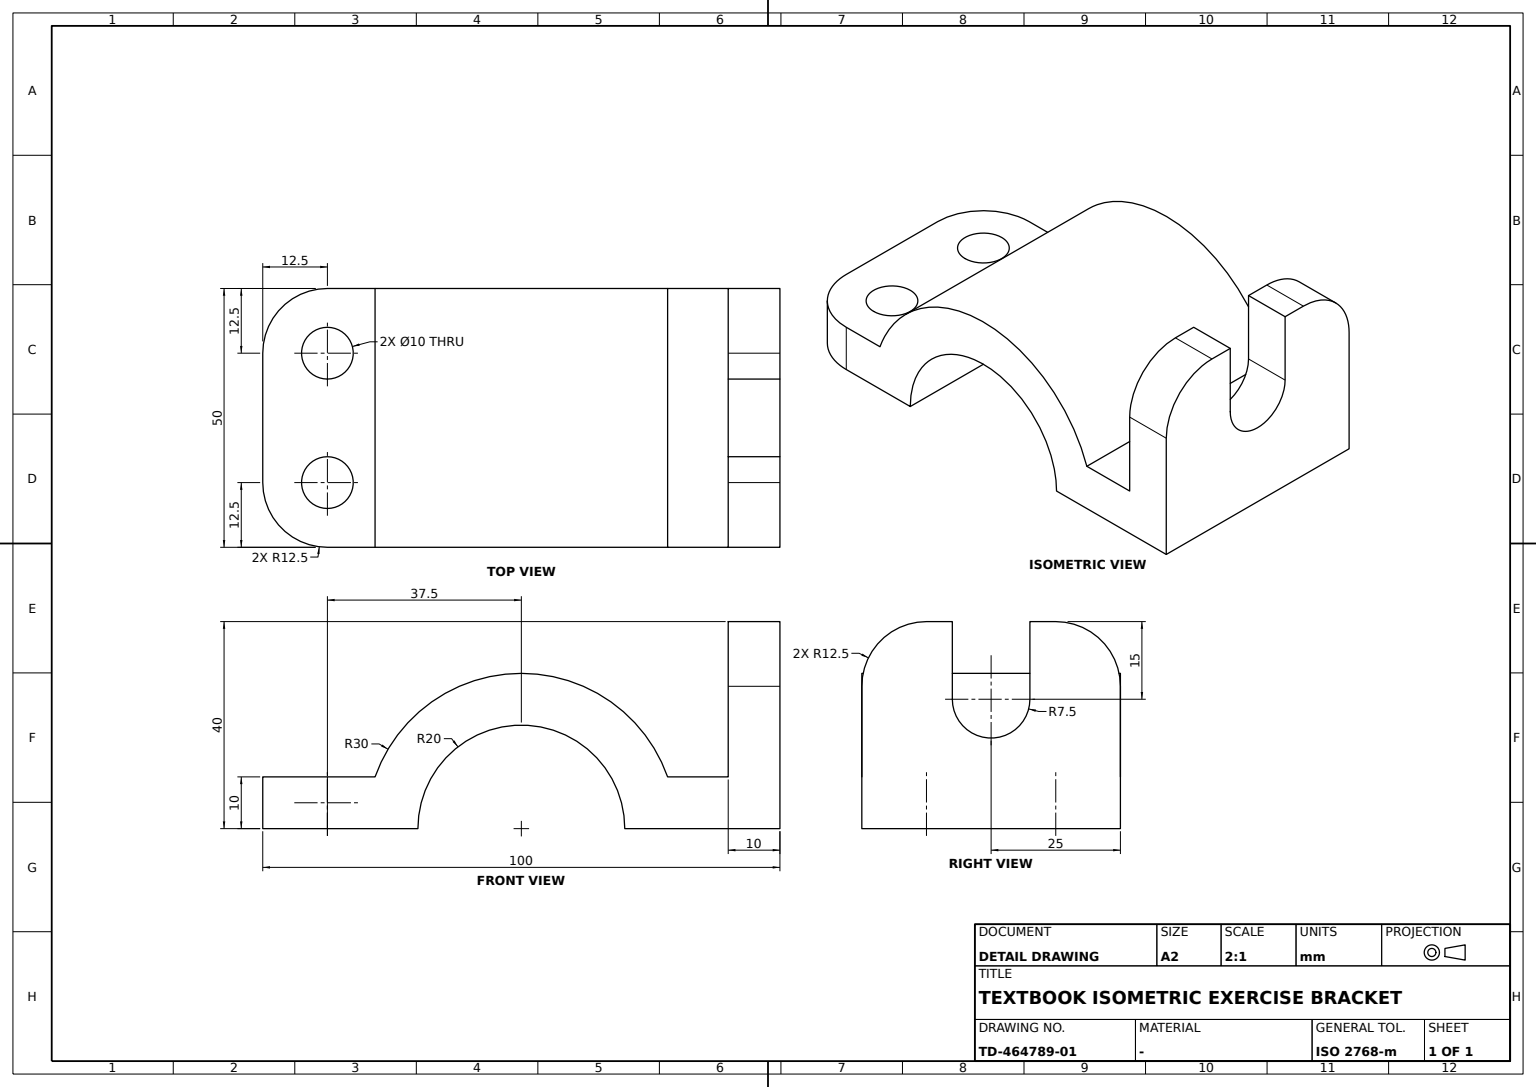
CATIA V5 part; units mm, degrees
sketch "Sketch1" plane through (0, 0, 0) normal (1, 0, 0) x (0, 1, 0)
  line L0 (-20, 0) -> (20, 0) construction
  point P0 (-20, 0)
  point P1 (20, 0)
  arc A0 (20, 0) -> (-20, 0) centre (0, 0) ccw
  point P2 (20, 0)
  point P3 (-20, 0)
  line L1 (20, 0) -> (50, 0)
  point P4 (50, 0)
  line L2 (-20, 0) -> (-50, 0)
  point P5 (-50, 0)
  line L3 (-50, 0) -> (-50, 10)
  arc A1 (28.2843, 10) -> (-28.2843, 10) centre (0, 0) ccw
  line L4 (20, 0) -> (30, 0) construction
  line L5 (-20, 0) -> (-30, 0) construction
  line L6 (-50, 10) -> (-28.2843, 10)
  line L7 (50, 0) -> (50, 40)
  line L8 (50, 40) -> (40, 40)
  line L9 (40, 40) -> (40, 10)
  point P6 (40, 10)
  line L10 (40, 10) -> (28.2843, 10)
  dimension "length L0" = 40
  dimension "distance P4 y axis" = 50
  dimension "distance P5 y axis" = 50
  dimension "length L3" = 10
  dimension "distance A0 A1" = 10
  dimension "length L7" = 40
  dimension "length L8" = 10
  dimension "distance P6 L1" = 10
  constraint midpoint L0 origin
  constraint horizontal L0 x-axis
  constraint horizontal L1 x-axis
  constraint horizontal L2 x-axis
  constraint horizontal L6 x-axis
  constraint horizontal L8 x-axis
  constraint horizontal L10 x-axis
  constraint coincidence A0 P0
  constraint coincidence P3 P0
  constraint coincidence L4 origin
  constraint coincidence L5 origin
  constraint coincidence P1 P2
  constraint vertical L3 y-axis
  constraint vertical L7 y-axis
  constraint vertical L9 y-axis
  constraint concentricity A0 A1
extrude "Pad1" add sketch "Sketch1" along normal mid plane 50
fillet "Fillet1" radius 12.5 1 edges at (25, 45, 40)
fillet "Fillet2" radius 12.5 1 edges at (-25, 45, 40)
fillet "Fillet3" radius 12.5 1 edges at (25, -50, 5)
fillet "Fillet4" radius 12.5 1 edges at (-25, -50, 5)
sketch "Sketch2" plane through (0, 0, 10) normal (0, 0, 1) x (1, 0, 0)
  circle A0 centre (-12.5, -37.5) radius 5
  arc A1 (-25, -37.5) -> (-12.5, -50) centre (-12.5, -37.5) ccw construction
  circle A2 centre (12.5, -37.5) radius 5
  arc A3 (12.5, -50) -> (25, -37.5) centre (12.5, -37.5) ccw construction
  dimension "radius A0" = 5
  dimension "radius A2" = 5
  constraint concentricity A0 A1
  constraint concentricity A2 A3
extrude "Pocket1" cut sketch "Sketch2" against normal blind 25
sketch "Sketch3" plane through (0, 50, 0) normal (0, 1, 0) x (-1, 0, 0)
  line L0 (-7.5, 40) -> (-7.5, 25)
  point P0 (-7.5, 40)
  point P1 (-7.5, 25)
  line L1 (25, 40) -> (-25, 40) construction
  line L2 (7.5, 40) -> (7.5, 25)
  point P2 (7.5, 40)
  point P3 (7.5, 25)
  arc A0 (-7.5, 25) -> (7.5, 25) centre (0, 25) ccw
  line L3 (-7.5, 40) -> (7.5, 40)
  dimension "distance L0 y axis" = 7.5
  dimension "distance P1 x axis" = 25
  dimension "distance P3 x axis" = 25
  dimension "distance L2 y axis" = 7.5
  constraint vertical L0 y-axis
  constraint vertical L2 y-axis
  constraint coincidence P0 L1
  constraint coincidence P2 L1
  constraint tangency A0 L2
  constraint horizontal L3 x-axis
extrude "Pocket2" cut sketch "Sketch3" against normal up to surface (10 mm away)
